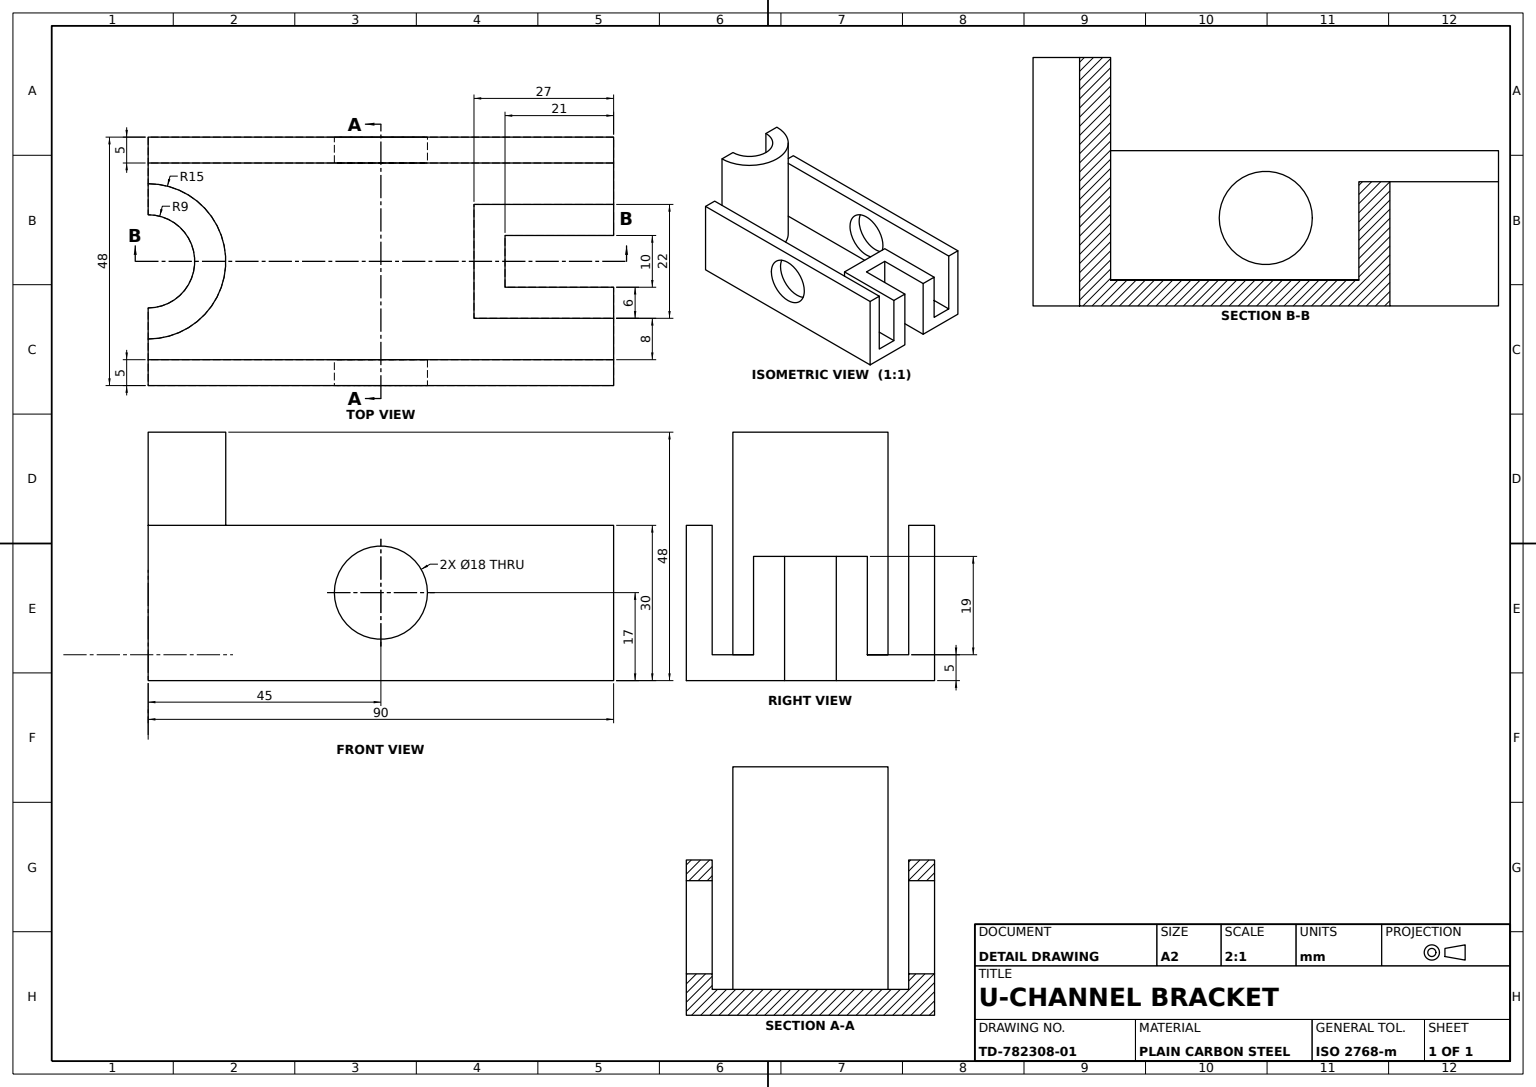
SolidWorks part; units mm, degrees
material "Plain Carbon Steel"
ref_plane "Front Plane" through (0, 0, 0) normal (0, 0, 1) x (1, 0, 0)
ref_plane "Top Plane" through (0, 0, 0) normal (0, 1, 0) x (1, 0, 0)
ref_plane "Right Plane" through (0, 0, 0) normal (1, 0, 0) x (0, 0, -1)
sketch "Base Block Sketch" plane through (0, 0, 0) normal (0, 1, 0) x (1, 0, 0)
  line L1 (-45, -24) -> (45, -24)
  line L2 (-45, -24) -> (-45, 24)
  line L3 (-45, 24) -> (45, 24)
  line L4 (45, -24) -> (45, 24)
  line L5 (-45, -24) -> (45, 24) construction
  line L6 (-45, 24) -> (45, -24) construction
  point P0 (0, 0)
  dimension "D1" = 48
  dimension "D2" = 90
extrude "Base Block 90x48x30" add sketch "Base Block Sketch" along normal blind 30
sketch "Channel Sketch" plane through (-45, 0, 0) normal (-1, 0, 0) x (0, 0, 1)
  line L0 (-24, 30) -> (24, 30) construction
  line L1 (-19, 30) -> (19, 30)
  line L2 (-19, 30) -> (-19, 5)
  line L3 (-19, 5) -> (19, 5)
  line L4 (19, 30) -> (19, 5)
  line L5 (-24, 30) -> (-24, 0) construction
  line L6 (24, 30) -> (24, 0) construction
  line L7 (-24, 0) -> (24, 0) construction
  dimension "D1" = 5
  dimension "D2" = 5
  dimension "D3" = 5
extrude "U-Channel Cut" cut sketch "Channel Sketch" against normal through all
sketch "Half Cylinder Post Sketch" plane through (0, 0, 0) normal (0, -1, 0) x (1, 0, 0)
  line L0 (-45, -24) -> (-45, 24) construction
  line L1 (-45, 15) -> (-45, -15)
  arc A0 (-45, -15) -> (-45, 15) centre (-45, 0) ccw
  dimension "D1" = 30
extrude "Half Cylinder Post Ø30" add sketch "Half Cylinder Post Sketch" against normal blind 48
sketch "Post Bore Sketch" plane through (0, 48, 0) normal (0, 1, 0) x (1, 0, 0)
  line L0 (-45, -15) -> (-45, 15) construction
  circle A0 centre (-45, 0) radius 9
  dimension "D1" = 18
extrude "Post Bore Ø18" cut sketch "Post Bore Sketch" against normal blind 48
sketch "End Tab Sketch" plane through (0, 5, 0) normal (0, 1, 0) x (1, 0, 0)
  line L0 (45, 19) -> (45, -19) construction
  line L1 (45, 11) -> (18, 11)
  line L2 (45, 11) -> (45, -11)
  line L3 (45, -11) -> (18, -11)
  line L4 (18, 11) -> (18, -11)
  line L5 (45, 19) -> (-45, 19) construction
  dimension "D1" = 27
  dimension "D2" = 22
  dimension "D3" = 8
extrude "End Tab" add sketch "End Tab Sketch" along normal blind 19
sketch "End Tab Slot Sketch" plane through (0, 24, 0) normal (0, 1, 0) x (1, 0, 0)
  line L0 (45, -11) -> (45, 11) construction
  line L1 (45, 5) -> (24, 5)
  line L2 (45, 5) -> (45, -5)
  line L3 (45, -5) -> (24, -5)
  line L4 (24, 5) -> (24, -5)
  line L5 (45, 11) -> (18, 11) construction
  dimension "D1" = 10
  dimension "D2" = 6
  dimension "D3" = 21
extrude "End Tab Slot" cut sketch "End Tab Slot Sketch" against normal through all
sketch "Side Hole Sketch" plane through (0, 0, 24) normal (0, 0, 1) x (1, 0, 0)
  line L0 (45, 30) -> (45, 0) construction
  line L1 (-45, 30) -> (45, 30) construction
  circle A0 centre (0, 17) radius 9
  dimension "D1" = 18
  dimension "D2" = 45
  dimension "D3" = 13
extrude "Side Hole Ø18" cut sketch "Side Hole Sketch" against normal blind 19
sketch "Opposite Side Hole Sketch" plane through (0, 0, -24) normal (0, 0, -1) x (-1, 0, 0)
  circle A1 centre (0, 17) radius 9
  circle A2 centre (0, 17) radius 9
  dimension "D1" = 0
extrude "Opposite Side Hole Ø18" cut sketch "Opposite Side Hole Sketch" against normal blind 19
